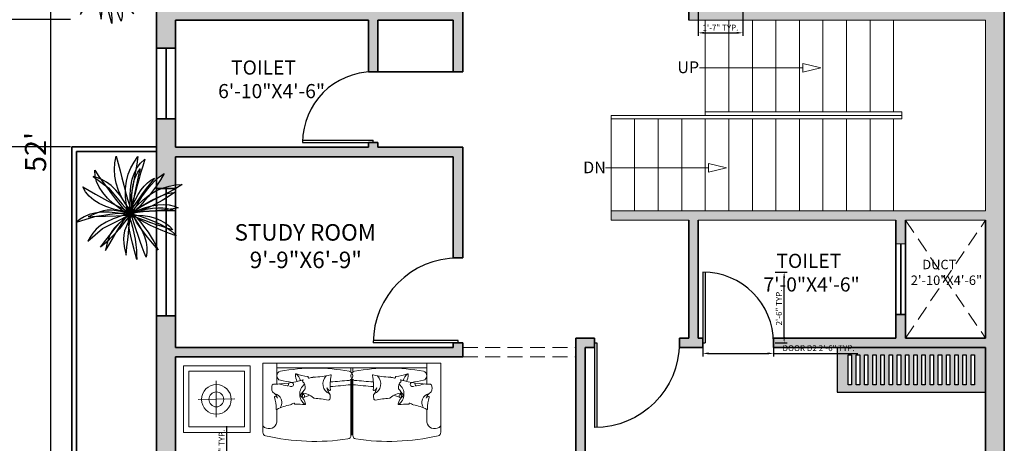
# Model space of a CAD drawing. Units: inches. Extents: x 1566 to 2546, y 1087 to 2705.
# Tile 18 of 27: x 2040 to 2458, y 1349 to 1529. Entities that reach past the tile are written whole.
import ezdxf

# ---------------------------------------------------------------- set-up
doc = ezdxf.new("R2010")
doc.units = ezdxf.units.IN
doc.linetypes.add('DASHED', pattern=[19.05, 12.7, -6.35])
for name, color, linetype, lineweight in [('A-ANNO-DIMS', 2, 'Continuous', 18), ('A-ANNO-TEXT', 7, 'Continuous', 18), ('A-AREA-IDEN', 7, 'Continuous', 18), ('A-DOOR', 4, 'Continuous', 25), ('A-FLOR-OVHD', 8, 'DASHED', 18), ('A-FLOR-STRS', 3, 'Continuous', 18), ('A-FURN', 8, 'Continuous', 18), ('A-WALL', 7, 'Continuous', 35), ('A-WALL-PATT', 8, 'Continuous', 13), ('L-PLNT', 94, 'Continuous', 18)]:
    doc.layers.add(name, color=color, linetype=linetype, lineweight=lineweight)
doc.layers.add('DIENHOA', color=3, linetype='Continuous')
doc.layers.add('MESA', color=7, linetype='Continuous')
doc.styles.get("Standard").update_dxf_attribs({"font": 'arial.ttf'})
doc.dimstyles.new('ISO-25', dxfattribs={"dimtxt": 2.5, "dimasz": 2.5, "dimexe": 1.25, "dimexo": 0.625, "dimtad": 1, "dimtxsty": 'Standard', "dimcen": 2.5, "dimadec": 0, "dimazin": 0, "dimtfac": 1, "dimtmove": 0, "dimatfit": 3, "dimfxl": 1, "dimarcsym": 0})

# ---------------------------------------------------------------- blocks, each defined once
blk = doc.blocks.new('*D3')
at = {"layer": 'A-ANNO-DIMS', "color": 0, "lineweight": -2, "transparency": 16777216}
for p, q in [((2061.66, 1784.43), (2052.02, 1784.43)), ((2053.27, 1781.93), (2053.27, 1162.93)), ((2061.66, 1160.43), (2052.02, 1160.43))]:
    blk.add_line(p, q, dxfattribs=at)
at = {"layer": 'A-ANNO-DIMS', "color": 0, "transparency": 16777216}
for points in [[(2052.85, 1781.93), (2053.69, 1781.93), (2053.27, 1784.43)], [(2052.85, 1162.93), (2053.69, 1162.93), (2053.27, 1160.43)]]:
    blk.add_solid(points, dxfattribs=at)
at = {"layer": 'Defpoints', "color": 0, "transparency": 16777216}
for p in [(2062.29, 1784.43), (2053.27, 1160.43), (2062.29, 1160.43)]:
    blk.add_point(p, dxfattribs=at)
at = {"layer": 'A-ANNO-DIMS', "color": 0, "transparency": 16777216, "insert": (2048.05, 1472.43), "char_height": 9, "attachment_point": 5, "rotation": 90}
blk.add_mtext("52'", dxfattribs=at)
blk = doc.blocks.new('d2')
for p, q in [((3364.08, 1632.29), (3364.08, 1602.29)), ((3365.08, 1632.29), (3365.08, 1602.29)), ((3364.08, 1602.29), (3365.08, 1602.29))]:
    blk.add_line(p, q)
at = {"ltscale": 0.3}
blk.add_arc((3364.08, 1602.29), 30, 0, 90, dxfattribs=at)
blk = doc.blocks.new('d1')
for p, q in [((3297.32, 1596.93), (3297.32, 1632.93)), ((3298.32, 1596.93), (3298.32, 1632.93)), ((3297.32, 1596.93), (3298.32, 1596.93))]:
    blk.add_line(p, q)
at = {"ltscale": 0.3}
blk.add_arc((3297.32, 1596.93), 36, 0, 90, dxfattribs=at)
blk = doc.blocks.new('Banco Lintz')
at = {"layer": 'MESA', "ltscale": 0.05}
h = blk.add_hatch(color=256, dxfattribs=at)
h.dxf.hatch_style = 1
h.set_gradient(color1=(138, 84, 66), color2=(0, 0, 0), one_color=1, name='INVCYLINDER')
h.paths.add_polyline_path([(0.48, 0), (0, 0), (0, -1.6), (0.48, -1.6)])
h.paths.add_polyline_path([(0.403, -0.509), (0.077, -0.509), (0.077, -0.472), (0.403, -0.472)], flags=16)
h.paths.add_polyline_path([(0.403, -0.561), (0.403, -0.597), (0.077, -0.597), (0.077, -0.561)], flags=16)
h.paths.add_polyline_path([(0.403, -0.421), (0.077, -0.421), (0.077, -0.384), (0.403, -0.384)], flags=16)
h.paths.add_polyline_path([(0.403, -0.649), (0.403, -0.686), (0.077, -0.686), (0.077, -0.649)], flags=16)
h.paths.add_polyline_path([(0.403, -0.332), (0.077, -0.332), (0.077, -0.296), (0.403, -0.296)], flags=16)
h.paths.add_polyline_path([(0.403, -0.737), (0.403, -0.774), (0.077, -0.774), (0.077, -0.737)], flags=16)
h.paths.add_polyline_path([(0.403, -0.244), (0.077, -0.244), (0.077, -0.207), (0.403, -0.207)], flags=16)
h.paths.add_polyline_path([(0.403, -0.826), (0.403, -0.863), (0.077, -0.863), (0.077, -0.826)], flags=16)
h.paths.add_polyline_path([(0.403, -0.156), (0.077, -0.156), (0.077, -0.119), (0.403, -0.119)], flags=16)
h.paths.add_polyline_path([(0.403, -0.914), (0.403, -0.951), (0.077, -0.951), (0.077, -0.914)], flags=16)
h.paths.add_polyline_path([(0.403, -1.003), (0.403, -1.039), (0.077, -1.039), (0.077, -1.003)], flags=16)
h.paths.add_polyline_path([(0.403, -1.091), (0.403, -1.128), (0.077, -1.128), (0.077, -1.091)], flags=16)
h.paths.add_polyline_path([(0.403, -1.179), (0.403, -1.216), (0.077, -1.216), (0.077, -1.179)], flags=16)
h.paths.add_polyline_path([(0.403, -1.268), (0.403, -1.304), (0.077, -1.304), (0.077, -1.268)], flags=16)
h.paths.add_polyline_path([(0.403, -1.356), (0.403, -1.393), (0.077, -1.393), (0.077, -1.356)], flags=16)
h.paths.add_polyline_path([(0.403, -1.444), (0.403, -1.481), (0.077, -1.481), (0.077, -1.444)], flags=16)
for points in [[(0, -1.6), (0.48, -1.6), (0.48, 0), (0, 0)], [(0.077, -0.119), (0.403, -0.119), (0.403, -0.156), (0.077, -0.156)], [(0.077, -0.207), (0.403, -0.207), (0.403, -0.244), (0.077, -0.244)], [(0.077, -0.296), (0.403, -0.296), (0.403, -0.332), (0.077, -0.332)], [(0.077, -0.384), (0.403, -0.384), (0.403, -0.421), (0.077, -0.421)], [(0.077, -0.472), (0.403, -0.472), (0.403, -0.509), (0.077, -0.509)], [(0.077, -0.561), (0.403, -0.561), (0.403, -0.597), (0.077, -0.597)], [(0.077, -0.649), (0.403, -0.649), (0.403, -0.686), (0.077, -0.686)], [(0.077, -0.737), (0.403, -0.737), (0.403, -0.774), (0.077, -0.774)], [(0.077, -0.826), (0.403, -0.826), (0.403, -0.863), (0.077, -0.863)], [(0.077, -0.914), (0.403, -0.914), (0.403, -0.951), (0.077, -0.951)], [(0.077, -1.003), (0.403, -1.003), (0.403, -1.039), (0.077, -1.039)], [(0.077, -1.091), (0.403, -1.091), (0.403, -1.128), (0.077, -1.128)], [(0.077, -1.179), (0.403, -1.179), (0.403, -1.216), (0.077, -1.216)], [(0.077, -1.268), (0.403, -1.268), (0.403, -1.304), (0.077, -1.304)], [(0.077, -1.356), (0.403, -1.356), (0.403, -1.393), (0.077, -1.393)], [(0.077, -1.444), (0.403, -1.444), (0.403, -1.481), (0.077, -1.481)]]:
    blk.add_lwpolyline(points, close=True, dxfattribs=at)
blk = doc.blocks.new('Cay03_mb')
at = {"layer": 'DIENHOA'}
for p, q in [((79, 504), (119, 555)), ((119, 555), (166, 599)), ((166, 599), (142, 519)), ((25, 374), (49, 444)), ((49, 444), (79, 504)), ((119, 442), (97, 366)), ((142, 519), (119, 442)), ((-365, 390), (-414, 403)), ((-414, 403), (-240, 278)), ((-315, 371), (-365, 390)), ((-264, 343), (-315, 371)), ((-211, 305), (-264, 343)), ((10, 295), (25, 374)), ((97, 366), (76, 291)), ((-240, 278), (-88, 95)), ((-158, 252), (-211, 305)), ((-104, 184), (-158, 252)), ((2, 206), (10, 295)), ((76, 291), (56, 216)), ((219, 200), (291, 243)), ((291, 243), (363, 275)), ((363, 275), (437, 297)), ((438, 231), (364, 193)), ((437, 297), (511, 310)), ((512, 271), (438, 231)), ((511, 310), (586, 314)), ((586, 314), (512, 271)), ((-50, 98), (-104, 184)), ((0, 105), (2, 206)), ((37, 142), (20, 68)), ((56, 216), (37, 142)), ((76, 75), (147, 144)), ((217, 117), (145, 77)), ((147, 144), (219, 200)), ((290, 155), (217, 117)), ((364, 193), (290, 155)), ((-345, 5), (-400, -17)), ((-299, 20), (-345, 5)), ((-255, 27), (-299, 20)), ((-208, 28), (-255, 27)), ((-153, 22), (-208, 28)), ((-83, 10), (-153, 22)), ((-88, 95), (5, -8)), ((5, -8), (-83, 10)), ((5, -8), (-50, 98)), ((5, -8), (0, 105)), ((5, -8), (76, 75)), ((20, 68), (5, -8)), ((75, 36), (5, -8)), ((5, -8), (100, 18)), ((46, 1), (5, -8)), ((97, 7), (46, 1)), ((145, 77), (75, 36)), ((155, 12), (97, 7)), ((100, 18), (182, 37)), ((220, 15), (155, 12)), ((182, 37), (253, 49)), ((289, 17), (220, 15)), ((253, 49), (315, 54)), ((362, 19), (289, 17)), ((315, 54), (369, 53)), ((436, 19), (362, 19)), ((369, 53), (419, 47)), ((419, 47), (465, 35)), ((510, 19), (436, 19)), ((465, 35), (510, 19)), ((-400, -17), (-468, -48)), ((-468, -48), (-376, -38)), ((-376, -38), (-295, -28)), ((-295, -28), (-226, -19)), ((-226, -19), (-166, -11)), ((-166, -11), (-114, -6)), ((-120, -122), (-80, -80)), ((-114, -6), (-69, -3)), ((-80, -80), (-45, -46)), ((-33, -69), (-75, -127)), ((-69, -3), (-30, -3)), ((-45, -46), (-17, -22)), ((5, -8), (-33, -69)), ((-30, -3), (5, -8)), ((-17, -22), (5, -8)), ((5, -8), (57, -73)), ((26, -64), (5, -8)), ((5, -8), (113, -40)), ((53, -42), (5, -8)), ((47, -126), (26, -64)), ((107, -76), (53, -42)), ((57, -73), (100, -139)), ((166, -110), (107, -76)), ((113, -40), (207, -74)), ((229, -143), (166, -110)), ((207, -74), (290, -108)), ((290, -108), (359, -141)), ((-216, -236), (-166, -174)), ((-166, -174), (-120, -122)), ((-118, -181), (-162, -231)), ((-75, -127), (-118, -181)), ((69, -191), (47, -126)), ((91, -257), (69, -191)), ((100, -139), (136, -204)), ((136, -204), (163, -268)), ((296, -175), (229, -143)), ((367, -205), (296, -175)), ((359, -141), (417, -174)), ((442, -233), (367, -205)), ((417, -174), (463, -204)), ((463, -204), (496, -232)), ((-330, -387), (-271, -307)), ((-250, -318), (-291, -355)), ((-271, -307), (-216, -236)), ((-206, -276), (-250, -318)), ((-162, -231), (-206, -276)), ((113, -322), (91, -257)), ((135, -386), (113, -322)), ((163, -268), (181, -330)), ((181, -330), (190, -390)), ((519, -258), (442, -233)), ((496, -232), (519, -258)), ((-291, -355), (-330, -387)), ((158, -445), (135, -386)), ((190, -390), (190, -446)), ((180, -499), (158, -445)), ((190, -446), (180, -499))]:
    blk.add_line(p, q, dxfattribs=at)
for points in [[(24, -5), (-41, 82), (-92, 167), (-130, 249), (-156, 330), (-170, 408), (-175, 484), (-170, 559), (-157, 633)], [(-157, 633), (-132, 551), (-111, 470), (-90, 389), (-70, 309), (-49, 229), (-27, 150), (-3, 72), (24, -5)], [(-16, -27), (-38, 80), (-49, 178), (-49, 269), (-39, 353), (-19, 430), (9, 501), (45, 567), (88, 629)], [(88, 629), (75, 544), (61, 461), (46, 379), (31, 298), (16, 217), (3, 136), (-8, 55), (-16, -27)], [(-396, 474), (-348, 406), (-301, 339), (-254, 275), (-208, 212), (-162, 151), (-115, 91), (-66, 32), (-16, -27)], [(-16, -27), (-108, 39), (-187, 102), (-252, 163), (-305, 224), (-345, 285), (-374, 347), (-390, 409), (-396, 474)], [(24, -5), (20, 93), (20, 177), (25, 249), (34, 310), (47, 363), (65, 409), (87, 452), (113, 492)], [(113, 492), (96, 420), (79, 347), (64, 276), (50, 208), (38, 145), (30, 87), (25, 36), (24, -5)], [(273, 387), (228, 329), (182, 270), (138, 212), (97, 156), (60, 103), (28, 55), (2, 11), (-16, -27)], [(-16, -27), (21, 64), (57, 140), (91, 203), (125, 255), (160, 297), (195, 332), (233, 362), (273, 387)], [(384, 437), (342, 368), (298, 302), (253, 239), (206, 181), (159, 127), (113, 78), (68, 34), (24, -5)], [(24, -5), (80, 92), (134, 176), (186, 248), (234, 309), (279, 357), (319, 395), (355, 421), (384, 437)], [(-530, 290), (-458, 248), (-388, 208), (-319, 169), (-251, 131), (-183, 95), (-115, 60), (-46, 26), (24, -5)], [(24, -5), (-87, 15), (-185, 40), (-270, 68), (-344, 101), (-406, 140), (-457, 184), (-499, 233), (-530, 290)], [(497, 224), (429, 178), (362, 137), (294, 99), (227, 66), (162, 37), (100, 11), (40, -10), (-16, -27)], [(-16, -27), (75, 38), (160, 92), (237, 136), (307, 170), (368, 195), (420, 213), (463, 222), (497, 224)], [(-16, -27), (-134, -5), (-235, 5), (-322, 5), (-396, -5), (-459, -22), (-512, -46), (-558, -74), (-598, -105)], [(24, -5), (99, 30), (173, 57), (245, 77), (313, 88), (378, 92), (438, 87), (493, 74), (541, 52)], [(541, 52), (484, 43), (421, 35), (354, 28), (285, 21), (216, 14), (148, 8), (83, 2), (24, -5)], [(-598, -105), (-393, -44), (-155, -37), (-16, -27)], [(-472, -320), (-310, -179), (-98, -73), (24, -5)], [(24, -5), (-92, -35), (-188, -68), (-267, -105), (-330, -145), (-380, -187), (-418, -231), (-448, -275), (-472, -320)], [(-276, -424), (-227, -345), (-186, -276), (-150, -216), (-119, -164), (-91, -120), (-66, -82), (-41, -52), (-16, -27)], [(-16, -27), (-85, -86), (-137, -133), (-176, -173), (-204, -210), (-226, -249), (-243, -295), (-258, -352), (-276, -424)], [(24, -5), (-14, -88), (-41, -153), (-60, -205), (-70, -251), (-73, -295), (-69, -344), (-60, -402), (-45, -475)], [(-45, -475), (-34, -383), (-25, -303), (-18, -233), (-12, -173), (-6, -121), (2, -77), (11, -39), (24, -5)], [(76, -524), (49, -428), (27, -342), (9, -264), (-4, -196), (-12, -138), (-17, -90), (-18, -53), (-16, -27)], [(478, -192), (422, -176), (361, -157), (298, -135), (232, -113), (167, -89), (102, -67), (41, -45), (-16, -27)], [(-16, -27), (67, -27), (146, -33), (219, -45), (286, -63), (346, -87), (398, -117), (443, -152), (478, -192)], [(-16, -27), (8, -95), (29, -163), (44, -231), (56, -296), (65, -359), (71, -419), (74, -474), (76, -524)], [(316, -418), (251, -343), (195, -273), (147, -210), (106, -154), (74, -105), (50, -63), (33, -30), (24, -5)], [(24, -5), (75, -57), (122, -111), (164, -165), (203, -219), (237, -273), (267, -324), (294, -373), (316, -418)]]:
    blk.add_lwpolyline(points, dxfattribs=at)
blk = doc.blocks.new('CUSHION-A')
blk.add_line((12.54, 5.91), (18.02, 5.91))
for centre, radius, start, end in [((0.45, 17.36), 0.472, 195.6578, 312.8337), ((-47.31, 3.98), 49.13, 0.5535, 15.4148), ((3.38, 14.21), 3.83, 84.2387, 132.8337), ((6.08, 20.97), 5.32, 217.6048, 326.1053), ((33.69, 53.65), 46.53, 229.9755, 234.1671), ((-41.81, -4.21), 52.85, 22.7112, 23.5018), ((11.64, 12), 6.29, 102.876, 140.0789), ((10.29, 17.91), 0.236, 351.7886, 102.876), ((10.29, 17.91), 0.236, 351.7886, 102.876), ((30.09, 15.05), 19.77, 171.7886, 183.7804), ((6.59, 16.12), 0.236, 234.1671, 341.1685), ((10.12, 13.26), 0.236, 89.311, 200.6915), ((18.72, 16.51), 9.43, 200.6915, 210.5832), ((10.12, 13.73), 0.236, 269.311, 3.7804), ((1.93, 11.97), 1.05, 232.8444, 267.2985), ((-19.11, 13.83), 21.87, 342.6177, 350.951), ((1.9, 11.4), 0.472, 267.2985, 277.3574), ((2.02, 10.46), 0.472, 350.951, 97.3574), ((30.09, 15.05), 19.77, 189.7298, 207.2752), ((2.2, 7.1), 0.472, 156.2045, 183.614), ((-47.31, 3.98), 49.13, 0.5535, 3.614), ((2.29, 4.45), 0.472, 180.5535, 248.334), ((4.84, 4.48), 0.472, 292.6623, 328.3929), ((9.43, 1.66), 4.91, 110.2155, 148.3929), ((7.3, 5.16), 0.236, 171.7015, 287.2637), ((8.61, 4.97), 1.56, 124.2109, 171.7015), ((12.04, -10.09), 15.74, 89.041, 107.2637), ((12.31, 5.88), 0.236, 269.041, 27.2752), ((17.28, 2.55), 3.44, 328.6411, 77.5888), ((3.54, 7.6), 3.85, 248.334, 292.6623), ((18.88, 1.57), 1.57, 270, 328.6411)]:
    blk.add_arc(centre, radius, start, end)
blk = doc.blocks.new('CUSHION-B')
for centre, radius, start, end in [((0.72, 14.91), 0.283, 77.7826, 196.0168), ((-22.35, 8.29), 23.73, 358.4714, 16.0168), ((4.78, 33.64), 18.88, 257.7826, 276.0053), ((5.1, 19.21), 5.89, 278.9571, 310.4913), ((5.29, 15.11), 1.87, 292.9525, 340.443), ((6.79, 14.58), 0.283, 340.443, 96.0053), ((9.49, 10.31), 4.45, 72.8696, 97.2038), ((69.07, 2.72), 58.96, 169.0518, 174.8479), ((10.63, 14.03), 0.567, 349.0518, 72.8696), ((-22.35, 8.29), 23.73, 340.5302, 352.522), ((1.45, 5.16), 0.283, 78.0525, 172.522), ((-9.32, 3.91), 11.32, 9.4331, 19.3248), ((1.57, 5.72), 0.283, 258.0525, 9.4331), ((16.33, 2.29), 8.16, 138.6039, 177.0681), ((9.79, 8.07), 0.567, 317.5655, 354.8479), ((0.28, 0.28), 0.283, 160.5302, 271.6176), ((3.81, -2.51), 4.68, 100.8696, 144.3073), ((0.08, 7.55), 7.55, 271.6176, 294.8398), ((2.15, 7.87), 7.94, 319.38, 328.0577), ((9.14, 2.07), 0.945, 40.8427, 147.338), ((9.41, 3.05), 0.814, 43.9174, 130.1627)]:
    blk.add_arc(centre, radius, start, end)
blk = doc.blocks.new('*D37')
at = {"layer": 'A-ANNO-DIMS', "color": 0, "lineweight": -2, "transparency": 16777216}
for p, q in [((2330.29, 1390.81), (2330.29, 1385.68)), ((2360.29, 1390.81), (2360.29, 1385.68)), ((2332.79, 1386.93), (2357.79, 1386.93)), ((2360.29, 1386.93), (2396.04, 1386.93))]:
    blk.add_line(p, q, dxfattribs=at)
at = {"layer": 'A-ANNO-DIMS', "color": 0, "transparency": 16777216}
for points in [[(2332.79, 1387.35), (2332.79, 1386.52), (2330.29, 1386.93)], [(2357.79, 1387.35), (2357.79, 1386.52), (2360.29, 1386.93)]]:
    blk.add_solid(points, dxfattribs=at)
at = {"layer": 'Defpoints', "color": 0, "transparency": 16777216}
for p in [(2330.29, 1391.43), (2360.29, 1391.43), (2360.29, 1386.93)]:
    blk.add_point(p, dxfattribs=at)
at = {"layer": 'A-ANNO-DIMS', "color": 0, "transparency": 16777216, "insert": (2379.41, 1388.85), "char_height": 2.5, "attachment_point": 5}
blk.add_mtext('DOOR D2 2\'-6" TYP.', dxfattribs=at)
blk = doc.blocks.new('*D38')
at = {"layer": 'A-ANNO-DIMS', "color": 0, "lineweight": -2, "transparency": 16777216}
for p, q in [((2360.91, 1421.43), (2366.04, 1421.43)), ((2364.79, 1393.93), (2364.79, 1418.93)), ((2360.91, 1391.43), (2366.04, 1391.43))]:
    blk.add_line(p, q, dxfattribs=at)
at = {"layer": 'A-ANNO-DIMS', "color": 0, "transparency": 16777216}
for points in [[(2364.37, 1418.93), (2365.21, 1418.93), (2364.79, 1421.43)], [(2364.37, 1393.93), (2365.21, 1393.93), (2364.79, 1391.43)]]:
    blk.add_solid(points, dxfattribs=at)
at = {"layer": 'Defpoints', "color": 0, "transparency": 16777216}
for p in [(2360.29, 1421.43), (2364.79, 1421.43), (2360.29, 1391.43)]:
    blk.add_point(p, dxfattribs=at)
at = {"layer": 'A-ANNO-DIMS', "color": 0, "transparency": 16777216, "insert": (2362.89, 1406.43), "char_height": 2.5, "attachment_point": 5, "rotation": 90}
blk.add_mtext('2\'-6" TYP.', dxfattribs=at)
blk = doc.blocks.new('*D42')
at = {"layer": 'A-ANNO-DIMS', "color": 0, "lineweight": -2, "transparency": 16777216}
for p, q in [((2328.29, 1531.81), (2328.29, 1521.73)), ((2347.19, 1531.81), (2347.19, 1521.73)), ((2330.79, 1522.98), (2344.69, 1522.98))]:
    blk.add_line(p, q, dxfattribs=at)
at = {"layer": 'A-ANNO-DIMS', "color": 0, "transparency": 16777216}
for points in [[(2330.79, 1523.4), (2330.79, 1522.57), (2328.29, 1522.98)], [(2344.69, 1523.4), (2344.69, 1522.57), (2347.19, 1522.98)]]:
    blk.add_solid(points, dxfattribs=at)
at = {"layer": 'Defpoints', "color": 0, "transparency": 16777216}
for p in [(2328.29, 1532.43), (2347.19, 1532.43), (2347.19, 1522.98)]:
    blk.add_point(p, dxfattribs=at)
at = {"layer": 'A-ANNO-DIMS', "color": 0, "transparency": 16777216, "insert": (2337.74, 1524.87), "char_height": 2.5, "attachment_point": 5}
blk.add_mtext('1\'-7" TYP.', dxfattribs=at)
blk = doc.blocks.new('*D55')
at = {"layer": 'A-ANNO-DIMS', "color": 0, "lineweight": -2, "transparency": 16777216}
for p, q in [((2128.15, 1316.53), (2128.15, 1356.06)), ((2126.37, 1316.53), (2129.4, 1316.53)), ((2128.15, 1302.98), (2128.15, 1314.03)), ((2126.37, 1300.48), (2129.4, 1300.48))]:
    blk.add_line(p, q, dxfattribs=at)
at = {"layer": 'A-ANNO-DIMS', "color": 0, "transparency": 16777216}
for points in [[(2127.74, 1314.03), (2128.57, 1314.03), (2128.15, 1316.53)], [(2127.74, 1302.98), (2128.57, 1302.98), (2128.15, 1300.48)]]:
    blk.add_solid(points, dxfattribs=at)
at = {"layer": 'Defpoints', "color": 0, "transparency": 16777216}
for p in [(2125.75, 1316.53), (2128.15, 1316.53), (2125.75, 1300.48)]:
    blk.add_point(p, dxfattribs=at)
at = {"layer": 'A-ANNO-DIMS', "color": 0, "transparency": 16777216, "insert": (2126.24, 1337.54), "char_height": 2.5, "attachment_point": 5, "rotation": 90}
blk.add_mtext('CUSHION C 1\'-4" TYP.', dxfattribs=at)
blk = doc.blocks.new('*D92')
at = {"layer": 'A-ANNO-DIMS', "color": 0, "lineweight": -2, "transparency": 16777216}
for p, q in [((2061.66, 1528.68), (2016.94, 1528.68)), ((2018.19, 1526.18), (2018.19, 1477.15)), ((2061.66, 1474.65), (2016.94, 1474.65))]:
    blk.add_line(p, q, dxfattribs=at)
at = {"layer": 'A-ANNO-DIMS', "color": 0, "transparency": 16777216}
for points in [[(2017.77, 1526.18), (2018.6, 1526.18), (2018.19, 1528.68)], [(2017.77, 1477.15), (2018.6, 1477.15), (2018.19, 1474.65)]]:
    blk.add_solid(points, dxfattribs=at)
at = {"layer": 'Defpoints', "color": 0, "transparency": 16777216}
for p in [(2062.29, 1528.68), (2018.19, 1474.65), (2062.29, 1474.65)]:
    blk.add_point(p, dxfattribs=at)
at = {"layer": 'A-ANNO-DIMS', "color": 0, "transparency": 16777216, "insert": (2016.29, 1501.66), "char_height": 2.5, "attachment_point": 5, "rotation": 90}
blk.add_mtext('4\'-6"', dxfattribs=at)

msp = doc.modelspace()

# ---------------------------------------------------------------- hatches: boundary and pattern name
at = {"layer": 'A-WALL-PATT'}
h = msp.add_hatch(color=256, dxfattribs=at)
h.dxf.hatch_style = 1
h.paths.add_polyline_path([(2106.29, 1385.43), (2228.29, 1385.43), (2228.29, 1391.43), (2224.29, 1391.43), (2224.29, 1389.43), (2106.29, 1389.43), (2106.29, 1402.93), (2098.29, 1402.93), (2098.29, 1343.43), (2106.29, 1343.43), (2106.29, 1347.74)], flags=17)
h.paths.add_polyline_path([(2106.29, 1259.43), (2098.29, 1259.43), (2098.29, 1209.43), (2155.29, 1209.43), (2155.29, 1217.43), (2143.41, 1217.43), (2106.29, 1217.43)], flags=17)
h.paths.add_polyline_path([(2334.29, 1217.43), (2280.29, 1217.43), (2280.29, 1389.43), (2284.29, 1389.43), (2284.29, 1391.43), (2284.29, 1393.43), (2276.29, 1393.43), (2276.29, 1217.43), (2227.29, 1217.43), (2227.29, 1209.43), (2334.29, 1209.43)], flags=17)
h.paths.add_polyline_path([(2106.29, 1486.43), (2098.29, 1486.43), (2098.29, 1460.88), (2099.11, 1461.64), (2100.44, 1462.65), (2101.57, 1463.26), (2099.97, 1460.62), (2098.29, 1458.1), (2098.29, 1456.93), (2100.35, 1456.93), (2100.77, 1457.12), (2103.56, 1457.95), (2106.29, 1458.4), (2106.29, 1470.43), (2224.29, 1470.43), (2224.29, 1427.43), (2228.29, 1427.43), (2228.29, 1474.43), (2192.29, 1474.43), (2192.29, 1476.43), (2188.29, 1476.43), (2188.29, 1474.43), (2106.29, 1474.43)], flags=17)
h.paths.add_polyline_path([(2106.29, 1585.43), (2192.29, 1585.43), (2192.29, 1589.43), (2098.29, 1589.43), (2098.29, 1573.93), (2106.29, 1573.93)], flags=17)
h.paths.add_polyline_path([(2228.29, 1585.43), (2232.29, 1585.43), (2232.29, 1589.43), (2224.29, 1589.43), (2222.29, 1589.43), (2222.29, 1585.43), (2224.29, 1585.43), (2224.29, 1532.43), (2106.29, 1532.43), (2106.29, 1543.93), (2098.29, 1543.93), (2098.29, 1516.43), (2106.29, 1516.43), (2106.29, 1528.43), (2188.29, 1528.43), (2188.29, 1506.43), (2192.29, 1506.43), (2192.29, 1528.43), (2224.29, 1528.43), (2224.29, 1506.43), (2228.29, 1506.43)], flags=17)
h.paths.add_polyline_path([(2106.29, 1680.43), (2098.29, 1680.43), (2098.29, 1625.43), (2106.29, 1625.43)], flags=17)
h.paths.add_polyline_path([(2458.29, 1784.43), (2098.29, 1784.43), (2098.29, 1776.43), (2276.29, 1776.43), (2276.29, 1589.43), (2268.29, 1589.43), (2268.29, 1585.43), (2280.29, 1585.43), (2280.29, 1652.43), (2284.29, 1652.43), (2284.29, 1656.43), (2280.29, 1656.43), (2280.29, 1776.43), (2398.29, 1776.43), (2398.29, 1746.43), (2402.29, 1746.43), (2402.29, 1776.43), (2450.29, 1776.43), (2450.29, 1532.43), (2375.49, 1532.43), (2328.29, 1532.43), (2328.29, 1612.43), (2324.29, 1612.43), (2324.29, 1528.43), (2450.29, 1528.43), (2450.29, 1447.43), (2291.29, 1447.43), (2291.29, 1443.43), (2324.29, 1443.43), (2324.29, 1393.43), (2320.29, 1393.43), (2320.29, 1389.43), (2330.29, 1389.43), (2330.29, 1393.43), (2328.29, 1393.43), (2328.29, 1443.43), (2412.29, 1443.43), (2412.29, 1433.43), (2416.29, 1433.43), (2416.29, 1443.43), (2450.29, 1443.43), (2450.29, 1393.43), (2416.29, 1393.43), (2416.29, 1403.43), (2412.29, 1403.43), (2412.29, 1393.43), (2360.29, 1393.43), (2360.29, 1389.43), (2450.29, 1389.43), (2450.29, 1217.43), (2396.29, 1217.43), (2396.29, 1209.43), (2450.29, 1209.43), (2450.29, 1136.43), (2458.29, 1136.43)])

# ---------------------------------------------------------------- linework, layer by layer
at = {"layer": 'A-FLOR-OVHD', "ltscale": 0.5}
for p, q in [((2416.29, 1443.43), (2450.29, 1393.43)), ((2416.29, 1393.43), (2450.29, 1443.43)), ((2228.29, 1389.43), (2276.29, 1389.43)), ((2228.29, 1385.43), (2276.29, 1385.43))]:
    msp.add_line(p, q, dxfattribs=at)
at = {"layer": 'A-FLOR-STRS'}
for p, q in [((2324.29, 1528.43), (2450.29, 1528.43)), ((2331.29, 1528.43), (2331.29, 1487.93)), ((2341.29, 1528.43), (2341.29, 1489.43)), ((2351.29, 1528.43), (2351.29, 1489.43)), ((2361.29, 1528.43), (2361.29, 1489.43)), ((2371.29, 1528.43), (2371.29, 1489.43)), ((2381.29, 1528.43), (2381.29, 1489.43)), ((2391.29, 1528.43), (2391.29, 1489.43)), ((2401.29, 1528.43), (2401.29, 1489.43)), ((2411.29, 1528.43), (2411.29, 1489.43)), ((2450.29, 1528.43), (2450.29, 1447.43)), ((2328.86, 1508.18), (2372.73, 1508.18)), ((2331.29, 1489.43), (2414.79, 1489.43)), ((2414.79, 1489.43), (2414.79, 1486.43)), ((2291.29, 1487.93), (2291.29, 1443.43)), ((2414.79, 1487.93), (2291.29, 1487.93)), ((2291.29, 1486.43), (2414.79, 1486.43)), ((2301.29, 1486.43), (2301.29, 1447.43)), ((2311.29, 1486.43), (2311.29, 1447.43)), ((2321.29, 1486.43), (2321.29, 1447.43)), ((2331.29, 1486.43), (2331.29, 1447.43)), ((2331.29, 1486.43), (2331.29, 1485.93)), ((2341.29, 1486.43), (2341.29, 1447.43)), ((2351.29, 1486.43), (2351.29, 1447.43)), ((2361.29, 1486.43), (2361.29, 1447.43)), ((2371.29, 1486.43), (2371.29, 1447.43)), ((2381.29, 1486.43), (2381.29, 1447.43)), ((2391.29, 1486.43), (2391.29, 1447.43)), ((2401.29, 1486.43), (2401.29, 1447.43)), ((2411.29, 1486.43), (2411.29, 1447.43)), ((2288.86, 1465.68), (2332.73, 1465.68)), ((2291.29, 1447.43), (2450.29, 1447.43)), ((2291.29, 1443.43), (2324.29, 1443.43)), ((2328.29, 1443.43), (2412.29, 1443.43)), ((2416.29, 1443.43), (2450.29, 1443.43)), ((2412.29, 1433.43), (2416.29, 1433.43))]:
    msp.add_line(p, q, dxfattribs=at)
for points in [[(2380.38, 1508.18), (2372.73, 1510.04), (2372.73, 1506.33)], [(2340.38, 1465.68), (2332.73, 1467.54), (2332.73, 1463.83)]]:
    msp.add_lwpolyline(points, close=True, dxfattribs=at)
at = {"layer": 'A-FURN'}
for p, q in [((2219, 1382.77), (2143.41, 1382.77)), ((2143.41, 1382.77), (2143.41, 1353.47)), ((2149.31, 1382.77), (2149.31, 1373.92)), ((2213.09, 1380.8), (2149.31, 1380.8)), ((2180.81, 1380.8), (2180.81, 1379.04)), ((2181.6, 1380.8), (2181.6, 1379.04)), ((2213.09, 1382.77), (2213.09, 1373.92)), ((2219, 1382.77), (2219, 1353.47)), ((2180.81, 1375.81), (2180.81, 1352.19)), ((2181.2, 1375.81), (2181.2, 1352.19)), ((2181.6, 1375.81), (2181.6, 1352.19)), ((2123.58, 1375.26), (2123.58, 1359.82)), ((2131.52, 1367.59), (2115.99, 1367.42))]:
    msp.add_line(p, q, dxfattribs=at)
for points in [[(2109.65, 1353.36), (2138, 1353.36), (2138, 1381.71), (2109.65, 1381.71)], [(2112.01, 1355.72), (2135.64, 1355.72), (2135.64, 1379.35), (2112.01, 1379.35)]]:
    msp.add_lwpolyline(points, close=True, dxfattribs=at)
for radius in [6.3, 3.15]:
    msp.add_circle((2123.67, 1367.42), radius, dxfattribs=at)
for centre, radius, start, end in [((2165.51, 1301.03), 79.67, 79.4658, 100.6108), ((2196.9, 1301.03), 79.67, 79.3892, 100.5342), ((2151.32, 1377.43), 1.97, 104.0803, 255.9197), ((2173.61, 1374.05), 4.71, 134.8494, 245.9788), ((2179.61, 1377.43), 1.98, 283.4421, 76.5579), ((2182.79, 1377.43), 1.98, 103.4421, 256.5579), ((2188.8, 1374.05), 4.71, 294.0212, 45.1506), ((2211.09, 1377.43), 1.97, 284.0803, 75.9197), ((2163.14, 1430.36), 56.2, 257.3591, 262.5789), ((2155.44, 1373.8), 0.999, 224.2238, 57.6435), ((2153.1, 1637.31), 265.11, 274.0948, 275.9995), ((2150.66, 1698.84), 324.68, 273.7815, 275.1985), ((2209.31, 1637.31), 265.11, 264.0005, 265.9052), ((2211.75, 1698.84), 324.68, 264.8015, 266.2185), ((2206.97, 1373.8), 0.999, 122.3565, 315.7762), ((2199.27, 1430.36), 56.2, 277.4211, 282.6409), ((2147.55, 1366.04), 3.93, 326.1078, 77.2372), ((2179.69, 1318.16), 53.54, 107.709, 111.2519), ((2182.72, 1318.16), 53.54, 68.7481, 72.291), ((2214.86, 1366.04), 3.93, 102.7628, 213.8922), ((2144.98, 1353.47), 1.57, 180, 255.2393), ((2165.54, 1444.39), 94.78, 257.2232, 278.4687), ((2179.24, 1352.19), 1.57, 279.7794, 0), ((2183.17, 1352.19), 1.57, 180, 260.2206), ((2196.86, 1444.39), 94.78, 261.5313, 282.7768), ((2217.42, 1353.47), 1.57, 284.7607, 0)]:
    msp.add_arc(centre, radius, start, end, dxfattribs=at)
at = {"layer": 'A-WALL'}
for p, q in [((2458.29, 1784.43), (2458.29, 1136.43)), ((2324.29, 1612.43), (2324.29, 1528.43)), ((2098.29, 1209.43), (2098.29, 1589.43)), ((2228.29, 1506.43), (2228.29, 1585.43)), ((2106.29, 1528.43), (2188.29, 1528.43)), ((2106.29, 1474.43), (2106.29, 1528.43)), ((2188.29, 1506.43), (2188.29, 1528.43)), ((2192.29, 1528.43), (2224.29, 1528.43)), ((2192.29, 1506.43), (2192.29, 1528.43)), ((2224.29, 1506.43), (2224.29, 1528.43)), ((2106.29, 1516.43), (2098.29, 1516.43)), ((2102.29, 1516.43), (2102.29, 1486.43)), ((2188.29, 1506.43), (2228.29, 1506.43)), ((2106.29, 1486.43), (2098.29, 1486.43)), ((2188.29, 1474.43), (2188.29, 1476.43)), ((2188.29, 1476.43), (2192.29, 1476.43)), ((2192.29, 1474.43), (2192.29, 1476.43)), ((2098.29, 1474.65), (2062.29, 1474.65)), ((2062.29, 1474.65), (2062.29, 1136.43)), ((2064.29, 1472.65), (2064.29, 1138.43)), ((2098.29, 1472.65), (2064.29, 1472.65)), ((2106.29, 1474.43), (2188.29, 1474.43)), ((2192.29, 1474.43), (2228.29, 1474.43)), ((2228.29, 1427.43), (2228.29, 1474.43)), ((2106.29, 1470.43), (2224.29, 1470.43)), ((2106.29, 1389.43), (2106.29, 1470.43)), ((2224.29, 1427.43), (2224.29, 1470.43)), ((2106.29, 1456.93), (2098.29, 1456.93)), ((2102.29, 1456.93), (2102.29, 1402.93)), ((2324.29, 1443.43), (2324.29, 1393.43)), ((2328.29, 1443.43), (2328.29, 1393.43)), ((2412.29, 1443.43), (2412.29, 1393.43)), ((2416.29, 1443.43), (2416.29, 1393.43)), ((2450.29, 1443.43), (2450.29, 1393.43)), ((2414.29, 1433.43), (2414.29, 1403.43)), ((2224.29, 1427.43), (2228.29, 1427.43)), ((2106.29, 1402.93), (2098.29, 1402.93)), ((2412.29, 1403.43), (2416.29, 1403.43)), ((2276.29, 1217.43), (2276.29, 1393.43)), ((2276.29, 1393.43), (2284.29, 1393.43)), ((2284.29, 1389.43), (2284.29, 1393.43)), ((2320.29, 1389.43), (2320.29, 1393.43)), ((2320.29, 1393.43), (2324.29, 1393.43)), ((2328.29, 1393.43), (2330.29, 1393.43)), ((2330.29, 1393.43), (2330.29, 1389.43)), ((2360.29, 1393.43), (2360.29, 1389.43)), ((2360.29, 1393.43), (2412.29, 1393.43)), ((2416.29, 1393.43), (2450.29, 1393.43)), ((2106.29, 1389.43), (2224.29, 1389.43)), ((2224.29, 1391.43), (2228.29, 1391.43)), ((2224.29, 1389.43), (2224.29, 1391.43)), ((2228.29, 1385.43), (2228.29, 1391.43)), ((2280.29, 1217.43), (2280.29, 1389.43)), ((2280.29, 1389.43), (2284.29, 1389.43)), ((2320.29, 1389.43), (2330.29, 1389.43)), ((2360.29, 1389.43), (2450.29, 1389.43)), ((2450.29, 1389.43), (2450.29, 1217.43)), ((2106.29, 1217.43), (2106.29, 1385.43)), ((2106.29, 1385.43), (2228.29, 1385.43))]:
    msp.add_line(p, q, dxfattribs=at)

# ---------------------------------------------------------------- block references
at = {"layer": 'A-DOOR', "rotation": 90}
for name, p in [('d2', (3792.58, -1887.65)), ('d1', (3823.22, -1905.89))]:
    msp.add_blockref(name, p, dxfattribs=at)
at = {"layer": 'A-DOOR'}
msp.add_blockref('d2', (-1033.79, -210.86), dxfattribs=at)
at = {"layer": 'A-DOOR', "xscale": -1, "rotation": 180}
msp.add_blockref('d1', (-1013.03, 2988.36), dxfattribs=at)
at = {"layer": 'A-FURN', "xscale": 39.3701, "yscale": 39.3701, "zscale": 39.3701, "rotation": 270}
msp.add_blockref('Banco Lintz', (2450.29, 1389.43), dxfattribs=at)
at = {"layer": 'A-FURN'}
for name, p, rotation in [('CUSHION-A', (2143.41, 1375.71), 270.0000000000012), ('CUSHION-B', (2157.26, 1378.29), 269.999999999994)]:
    msp.add_blockref(name, p, dxfattribs=dict(at, rotation=rotation))
at = {"layer": 'A-FURN', "extrusion": (0, 0, -1), "zscale": -1}
for name, p, rotation in [('CUSHION-B', (-2205.15, 1378.29), 269.9999999999944), ('CUSHION-A', (-2219, 1375.71), 269.9999999999992)]:
    msp.add_blockref(name, p, dxfattribs=dict(at, rotation=rotation))
at = {"layer": 'L-PLNT', "xscale": 0.0378941924884598, "yscale": 0.0378941924884598, "zscale": 0.0378941924884598}
for p in [(2076.46, 1546.83), (2087, 1446.68)]:
    msp.add_blockref('Cay03_mb', p, dxfattribs=at)

# ---------------------------------------------------------------- texts
at = {"layer": 'A-ANNO-TEXT'}
for s, p in [('UP', (2319.44, 1505.88)), ('DN', (2279.44, 1463.38))]:
    msp.add_text(s, height=5, dxfattribs=at).set_placement(p)
at = {"layer": 'A-AREA-IDEN', "attachment_point": 1}
for s, insert, char_height in [('   TOILET\\P6\'-10"X4\'-6"', (2124.42, 1511.26), 6), ('STUDY ROOM\\P   9\'-9"X6\'-9"', (2131.4, 1441.8), 7), ('   TOILET\\P7\'-0"X4\'-6"', (2356.01, 1429.21), 6), ('    DUCT\\P2\'-10"X4\'-6"', (2418.59, 1426.66), 4)]:
    msp.add_mtext_dynamic_manual_height_columns(s, width=111.7553, gutter_width=12.5, heights=[0], dxfattribs=dict(at, insert=insert, char_height=char_height))

# ---------------------------------------------------------------- dimensions: what is measured, and where the dimension line sits
at = {"layer": 'A-ANNO-DIMS'}
for base, p1, p2, override, picture, middle in [((2053.27, 1160.43), (2062.29, 1784.43), (2062.29, 1160.43), {"dimtxt": 9, "dimdec": 1, "dimlunit": 3, "dimclrd": 0, "dimclre": 0, "dimclrt": 0, "dimtdec": 1}, '*D3', (2048.05, 1472.43)), ((2018.19, 1474.65), (2062.29, 1528.68), (2062.29, 1474.65), {"dimdec": 1, "dimlfac": 1, "dimrnd": 0, "dimzin": 1, "dimdsep": 46, "dimlunit": 4, "dimfrac": 2}, '*D92', (2016.29, 1501.66))]:
    dim = msp.add_linear_dim(base=base, p1=p1, p2=p2, angle=90, dimstyle='ISO-25', override=override, dxfattribs=at)
    dim.commit()
    dim.dimension.update_dxf_attribs({"geometry": picture, "text_midpoint": middle})
for base, p1, p2, text, picture, middle in [((2347.19, 1522.98), (2328.29, 1532.43), (2347.19, 1532.43), '<> TYP.', '*D42', (2337.74, 1524.87)), ((2360.29, 1386.93), (2330.29, 1391.43), (2360.29, 1391.43), 'DOOR D2 <> TYP.', '*D37', (2379.41, 1388.85))]:
    dim = msp.add_linear_dim(base=base, p1=p1, p2=p2, text=text, dimstyle='ISO-25', override={"dimdec": 1, "dimrnd": 0, "dimzin": 1, "dimlunit": 4, "dimfrac": 2}, dxfattribs=at)
    dim.commit()
    dim.dimension.update_dxf_attribs({"geometry": picture, "text_midpoint": middle})
for base, p1, p2, text, picture, middle in [((2364.79, 1421.43), (2360.29, 1391.43), (2360.29, 1421.43), '<> TYP.', '*D38', (2362.89, 1406.43)), ((2128.1548, 1316.5307), (2125.7469, 1300.4777), (2125.7469, 1316.5307), 'CUSHION C <> TYP.', '*D55', (2126.2364, 1337.5445))]:
    dim = msp.add_linear_dim(base=base, p1=p1, p2=p2, angle=90, text=text, dimstyle='ISO-25', override={"dimdec": 1, "dimrnd": 0, "dimzin": 1, "dimlunit": 4, "dimfrac": 2}, dxfattribs=at)
    dim.commit()
    dim.dimension.update_dxf_attribs({"geometry": picture, "text_midpoint": middle})

doc.saveas('drawing.dxf')
